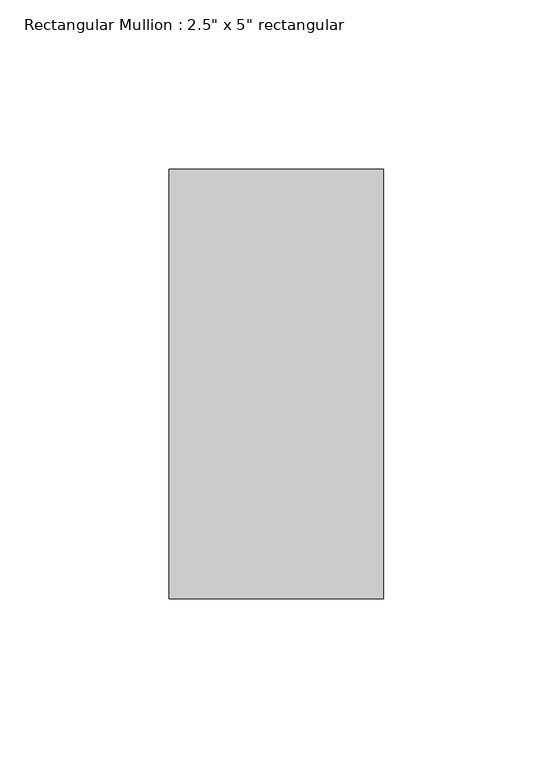
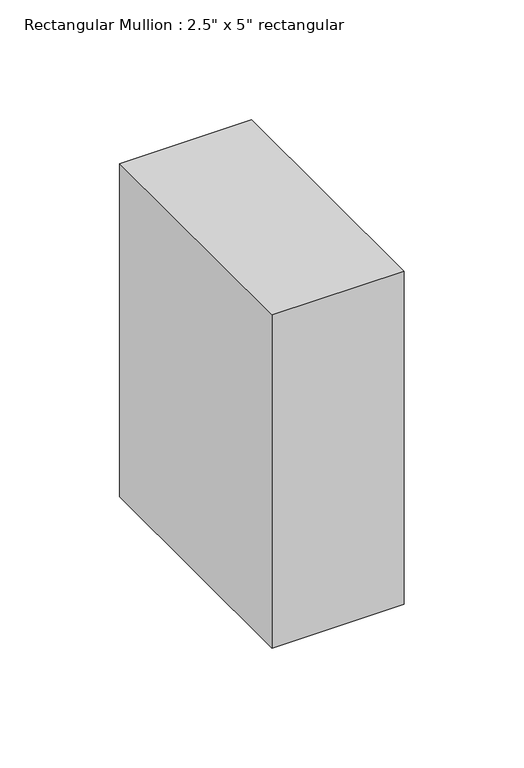
"""IFC4 building model written with IfcOpenShell, lengths in millimetres: member geometry."""

from ifc_helpers import new_model, si_unit, frame, origin, place, context, project, spatial, polyline, outline, extrude, source, transform, mapped, element, save


def member_4e7e4155(model_context):
    return source(origin(), model_context, "Body", "SweptSolid", [
        extrude(outline(polyline([(31.75, 63.5), (31.75, -63.5), (-31.75, -63.5), (-31.75, 63.5), (31.75, 63.5)])), frame((0.0, 0.0, -169.4874164), z_axis=(0.0, 0.0, 1.0), x_axis=(1.0, 0.0, 0.0)), (0.0, 0.0, 1.0), 169.4874164),
    ])


if __name__ == "__main__":
    model = new_model("IFC4")
    model_context = context("Model", 3, world=origin())
    ifc_project = project(units=[si_unit("LENGTHUNIT", "METRE", prefix="MILLI")], contexts=[model_context])
    site = spatial("IfcSite", under=ifc_project)
    building = spatial("IfcBuilding", under=site)
    placement = place(None, origin())
    member_shape = member_4e7e4155(model_context)
    element("IfcMember", 1, ObjectType="Rectangular Mullion : 2.5\" x 5\" rectangular", at=placement, inside=building, context=model_context, shape_type="MappedRepresentation", body=[
        mapped(member_shape, transform((0.0, 0.0, 0.0), x_axis=(1.0, 0.0, 0.0), y_axis=(0.0, 1.0, 0.0), z_axis=(0.0, 0.0, 1.0))),
    ])
    save(model, "model.ifc")

# Revit data of these elements
# Type "Rectangular Mullion : 2.5\" x 5\" rectangular"
#   built-in parameter 1007304 = 0.416667 (stored number, unit not read)
#   built-in parameter 1007301 = 0.104167 (stored number, unit not read)
#   built-in parameter 1007300 = 0.104167 (stored number, unit not read)
# Element 1 (IfcMember, "Rectangular Mullion : 2.5\" x 5\" rectangular")
#   Materials on its faces: "Aluminum"
# Materials
#   "Aluminum": class "Metal", colour RGB 247 247 247, transparency 0, Description = "Aluminum 6061", Cost = 0
